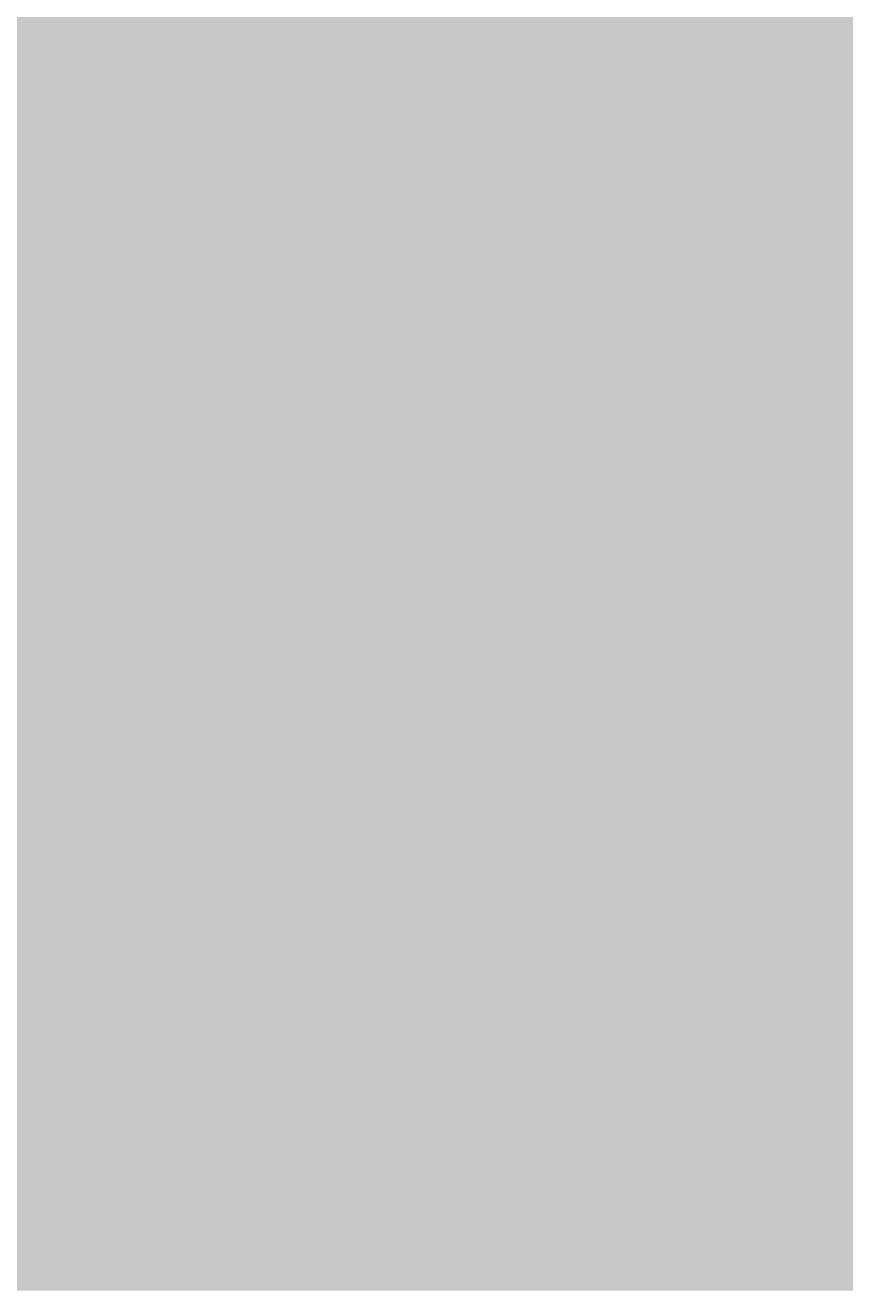
# Model space of a CAD drawing. Units: inches. Extents: x 84 to 1044, y -280 to 906.
# Tile 81 of 105: x 815 to 831, y 400 to 425. Entities that reach past the tile are written whole.
import ezdxf

# ---------------------------------------------------------------- set-up
doc = ezdxf.new("R2010")
doc.units = ezdxf.units.IN
doc.layers.add('A-ANNO-DIMS', color=2, linetype='Continuous', lineweight=18)
doc.layers.add('L-PLNT-PATT', color=9, linetype='Continuous', lineweight=9, true_color=0xafd9aa)
doc.styles.get("Standard").update_dxf_attribs({"font": 'arial.ttf'})
doc.dimstyles.get("Standard").update_dxf_attribs({"dimtxt": 0.18, "dimasz": 0.18, "dimexe": 0.18, "dimexo": 0.0625, "dimgap": 0.09, "dimtad": 0, "dimtih": 1, "dimtoh": 1, "dimdec": 4, "dimzin": 0, "dimdsep": 46, "dimtxsty": 'Standard', "dimcen": 0.09, "dimadec": 0, "dimazin": 0, "dimtfac": 1, "dimtdec": 4, "dimtofl": 0, "dimtmove": 0, "dimatfit": 3, "dimfxl": 1, "dimtolj": 1, "dimtzin": 0, "dimarcsym": 0})

# ---------------------------------------------------------------- blocks, each defined once
blk = doc.blocks.new('*D62')
at = {"layer": 'A-ANNO-DIMS', "color": 0, "lineweight": -2, "transparency": 16777216}
for p, q in [((203.179, 709.183), (203.179, 905.9)), ((896.074, 400.183), (896.074, 905.9)), ((203.359, 905.72), (549.232, 905.72)), ((895.894, 905.72), (550.021, 905.72))]:
    blk.add_line(p, q, dxfattribs=at)
at = {"layer": 'A-ANNO-DIMS', "color": 0, "transparency": 16777216}
for points in [[(203.359, 905.75), (203.359, 905.69), (203.179, 905.72)], [(895.894, 905.75), (895.894, 905.69), (896.074, 905.72)]]:
    blk.add_solid(points, dxfattribs=at)
at = {"layer": 'Defpoints', "color": 0, "transparency": 16777216}
for p in [(896.074, 905.72), (203.179, 709.12), (896.074, 400.12)]:
    blk.add_point(p, dxfattribs=at)
at = {"layer": 'A-ANNO-DIMS', "color": 0, "transparency": 16777216, "insert": (549.627, 905.72), "char_height": 0.18, "attachment_point": 5}
blk.add_mtext('\\A1;692.9', dxfattribs=at)

msp = doc.modelspace()

# ---------------------------------------------------------------- hatches: boundary and pattern name
at = {"layer": 'L-PLNT-PATT', "transparency": 33554597}
h = msp.add_hatch(color=256, dxfattribs=at)
h.dxf.hatch_style = 1
h.paths.add_polyline_path([(896.074, 511.12), (704.074, 511.12), (704.074, 491.62), (704.074, 419.62), (704.074, 400.12), (833.074, 400.12), (896.074, 400.12)])

# ---------------------------------------------------------------- dimensions: what is measured, and where the dimension line sits
at = {"layer": 'A-ANNO-DIMS'}
dim = msp.add_linear_dim(base=(896.074, 905.72), p1=(203.179, 709.12), p2=(896.074, 400.12), dimstyle='Standard', override={"dimdec": 1, "dimlfac": 1, "dimrnd": 0, "dimzin": 0, "dimdsep": 46, "dimlunit": 2}, dxfattribs=at)
dim.commit()
dim.dimension.update_dxf_attribs({"geometry": '*D62', "text_midpoint": (549.627, 905.72)})

doc.saveas('drawing.dxf')
